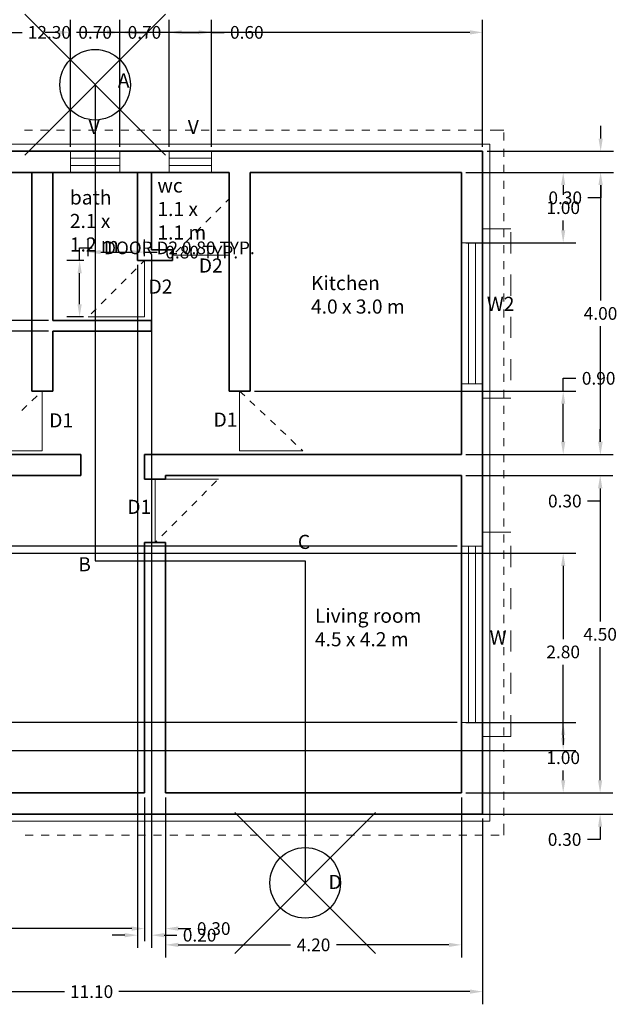
# Model space of a CAD drawing. Units: metres. Extents: x 37.9 to 70.9, y 22.7 to 44.8.
# Tile 2 of 4: x 44.9 to 53.4, y 22.7 to 36.7. Entities that reach past the tile are written whole.
import ezdxf

# ---------------------------------------------------------------- set-up
doc = ezdxf.new("R2010")
doc.units = ezdxf.units.M
doc.header["$LTSCALE"] = 50
doc.header["$MEASUREMENT"] = 0
doc.header["$PDMODE"] = 35
doc.header["$PDSIZE"] = -2
doc.linetypes.add('ACAD_ISO03W100', pattern=[30, 12, -18])
for name, color, linetype, lineweight in [('A-ANNO-DIMS', 2, 'Continuous', 18), ('A-ANNO-SYMB', 3, 'Continuous', 25), ('A-ANNO-TEXT', 7, 'Continuous', 18), ('A-AREA-IDEN', 7, 'Continuous', 18), ('A-DOOR', 4, 'Continuous', 18), ('A-FLOR-PLIN', 7, 'Continuous', 18), ('A-GLAZ', 4, 'Continuous', 18), ('A-ROOF-OVHD', 8, 'ACAD_ISO03W100', 13), ('A-WALL', 7, 'Continuous', 35)]:
    doc.layers.add(name, color=color, linetype=linetype, lineweight=lineweight)
doc.styles.get("Standard").update_dxf_attribs({"font": 'arial.ttf'})
doc.dimstyles.get("Standard").update_dxf_attribs({"dimtxt": 0.18, "dimasz": 0.18, "dimexe": 0.18, "dimexo": 0.0625, "dimgap": 0.09, "dimtad": 0, "dimtih": 1, "dimtoh": 1, "dimzin": 0, "dimdsep": 46, "dimtxsty": 'Standard', "dimcen": 0.09, "dimadec": 0, "dimazin": 0, "dimtfac": 1, "dimtofl": 0, "dimtmove": 0, "dimatfit": 3, "dimfxl": 1, "dimtolj": 1, "dimtzin": 0, "dimarcsym": 0})

# ---------------------------------------------------------------- blocks, each defined once
blk = doc.blocks.new('*D1')
at = {"layer": 'A-ANNO-DIMS', "color": 0, "linetype": 'ACAD_ISO03W100', "lineweight": -2, "transparency": 16777216}
for p, q in [((53.175, 34.98), (53.175, 35.16)), ((53.175, 34.32), (53.175, 34.14)), ((53.175, 34.14), (52.995, 34.14))]:
    blk.add_line(p, q, dxfattribs=at)
at = {"layer": 'A-ANNO-DIMS', "color": 0, "lineweight": -2, "transparency": 16777216}
for p, q in [((51.563, 34.8), (53.355, 34.8)), ((51.563, 34.5), (53.355, 34.5))]:
    blk.add_line(p, q, dxfattribs=at)
at = {"layer": 'A-ANNO-DIMS', "color": 0, "transparency": 16777216}
for points in [[(53.145, 34.98), (53.205, 34.98), (53.175, 34.8)], [(53.145, 34.32), (53.205, 34.32), (53.175, 34.5)]]:
    blk.add_solid(points, dxfattribs=at)
at = {"layer": 'Defpoints', "color": 0, "transparency": 16777216}
for p in [(51.5, 34.8), (51.5, 34.5), (53.175, 34.5)]:
    blk.add_point(p, dxfattribs=at)
at = {"layer": 'A-ANNO-DIMS', "color": 0, "transparency": 16777216, "insert": (52.672, 34.14), "char_height": 0.18, "attachment_point": 5}
blk.add_mtext('\\A1;0.30', dxfattribs=at)
blk = doc.blocks.new('*D2')
at = {"layer": 'A-ANNO-DIMS', "color": 0, "lineweight": -2, "transparency": 16777216}
for p, q in [((51.263, 34.5), (53.353, 34.5)), ((51.263, 30.5), (53.353, 30.5))]:
    blk.add_line(p, q, dxfattribs=at)
at = {"layer": 'A-ANNO-DIMS', "color": 0, "linetype": 'ACAD_ISO03W100', "lineweight": -2, "transparency": 16777216}
for p, q in [((53.173, 34.32), (53.173, 32.682)), ((53.173, 30.68), (53.173, 32.318))]:
    blk.add_line(p, q, dxfattribs=at)
at = {"layer": 'A-ANNO-DIMS', "color": 0, "transparency": 16777216}
for points in [[(53.143, 34.32), (53.203, 34.32), (53.173, 34.5)], [(53.143, 30.68), (53.203, 30.68), (53.173, 30.5)]]:
    blk.add_solid(points, dxfattribs=at)
at = {"layer": 'Defpoints', "color": 0, "transparency": 16777216}
for p in [(51.2, 34.5), (51.2, 30.5), (53.173, 30.5)]:
    blk.add_point(p, dxfattribs=at)
at = {"layer": 'A-ANNO-DIMS', "color": 0, "transparency": 16777216, "insert": (53.173, 32.5), "char_height": 0.18, "attachment_point": 5}
blk.add_mtext('\\A1;4.00', dxfattribs=at)
blk = doc.blocks.new('*D3')
at = {"layer": 'A-ANNO-DIMS', "color": 0, "linetype": 'ACAD_ISO03W100', "lineweight": -2, "transparency": 16777216}
for p, q in [((53.169, 30.68), (53.169, 30.86)), ((53.169, 30.02), (53.169, 29.84)), ((53.169, 29.84), (52.989, 29.84))]:
    blk.add_line(p, q, dxfattribs=at)
at = {"layer": 'A-ANNO-DIMS', "color": 0, "lineweight": -2, "transparency": 16777216}
for p, q in [((51.263, 30.5), (53.349, 30.5)), ((51.263, 30.2), (53.349, 30.2))]:
    blk.add_line(p, q, dxfattribs=at)
at = {"layer": 'A-ANNO-DIMS', "color": 0, "transparency": 16777216}
for points in [[(53.139, 30.68), (53.199, 30.68), (53.169, 30.5)], [(53.139, 30.02), (53.199, 30.02), (53.169, 30.2)]]:
    blk.add_solid(points, dxfattribs=at)
at = {"layer": 'Defpoints', "color": 0, "transparency": 16777216}
for p in [(51.2, 30.5), (51.2, 30.2), (53.169, 30.2)]:
    blk.add_point(p, dxfattribs=at)
at = {"layer": 'A-ANNO-DIMS', "color": 0, "transparency": 16777216, "insert": (52.666, 29.84), "char_height": 0.18, "attachment_point": 5}
blk.add_mtext('\\A1;0.30', dxfattribs=at)
blk = doc.blocks.new('*D4')
at = {"layer": 'A-ANNO-DIMS', "color": 0, "lineweight": -2, "transparency": 16777216}
for p, q in [((51.263, 30.2), (53.347, 30.2)), ((51.263, 25.7), (53.347, 25.7))]:
    blk.add_line(p, q, dxfattribs=at)
at = {"layer": 'A-ANNO-DIMS', "color": 0, "linetype": 'ACAD_ISO03W100', "lineweight": -2, "transparency": 16777216}
for p, q in [((53.167, 30.02), (53.167, 28.132)), ((53.167, 25.88), (53.167, 27.768))]:
    blk.add_line(p, q, dxfattribs=at)
at = {"layer": 'A-ANNO-DIMS', "color": 0, "transparency": 16777216}
for points in [[(53.137, 30.02), (53.197, 30.02), (53.167, 30.2)], [(53.137, 25.88), (53.197, 25.88), (53.167, 25.7)]]:
    blk.add_solid(points, dxfattribs=at)
at = {"layer": 'Defpoints', "color": 0, "transparency": 16777216}
for p in [(51.2, 30.2), (51.2, 25.7), (53.167, 25.7)]:
    blk.add_point(p, dxfattribs=at)
at = {"layer": 'A-ANNO-DIMS', "color": 0, "transparency": 16777216, "insert": (53.167, 27.95), "char_height": 0.18, "attachment_point": 5}
blk.add_mtext('\\A1;4.50', dxfattribs=at)
blk = doc.blocks.new('*D5')
at = {"layer": 'A-ANNO-DIMS', "color": 0, "linetype": 'ACAD_ISO03W100', "lineweight": -2, "transparency": 16777216}
for p, q in [((53.167, 25.88), (53.167, 26.06)), ((53.167, 25.22), (53.167, 25.04)), ((53.167, 25.04), (52.987, 25.04))]:
    blk.add_line(p, q, dxfattribs=at)
at = {"layer": 'A-ANNO-DIMS', "color": 0, "lineweight": -2, "transparency": 16777216}
for p, q in [((51.263, 25.7), (53.347, 25.7)), ((51.263, 25.4), (53.347, 25.4))]:
    blk.add_line(p, q, dxfattribs=at)
at = {"layer": 'A-ANNO-DIMS', "color": 0, "transparency": 16777216}
for points in [[(53.137, 25.88), (53.197, 25.88), (53.167, 25.7)], [(53.137, 25.22), (53.197, 25.22), (53.167, 25.4)]]:
    blk.add_solid(points, dxfattribs=at)
at = {"layer": 'Defpoints', "color": 0, "transparency": 16777216}
for p in [(51.2, 25.7), (51.2, 25.4), (53.167, 25.4)]:
    blk.add_point(p, dxfattribs=at)
at = {"layer": 'A-ANNO-DIMS', "color": 0, "transparency": 16777216, "insert": (52.663, 25.04), "char_height": 0.18, "attachment_point": 5}
blk.add_mtext('\\A1;0.30', dxfattribs=at)
blk = doc.blocks.new('*D6')
at = {"layer": 'A-ANNO-DIMS', "color": 0, "lineweight": -2, "transparency": 16777216}
for p, q in [((40.7, 25.637), (40.7, 23.597)), ((46.7, 25.637), (46.7, 23.597))]:
    blk.add_line(p, q, dxfattribs=at)
at = {"layer": 'A-ANNO-DIMS', "color": 0, "linetype": 'ACAD_ISO03W100', "lineweight": -2, "transparency": 16777216}
for p, q in [((40.88, 23.777), (43.376, 23.777)), ((46.52, 23.777), (44.024, 23.777))]:
    blk.add_line(p, q, dxfattribs=at)
at = {"layer": 'A-ANNO-DIMS', "color": 0, "transparency": 16777216}
for points in [[(40.88, 23.807), (40.88, 23.747), (40.7, 23.777)], [(46.52, 23.807), (46.52, 23.747), (46.7, 23.777)]]:
    blk.add_solid(points, dxfattribs=at)
at = {"layer": 'Defpoints', "color": 0, "transparency": 16777216}
for p in [(40.7, 25.7), (46.7, 25.7), (46.7, 23.777)]:
    blk.add_point(p, dxfattribs=at)
at = {"layer": 'A-ANNO-DIMS', "color": 0, "transparency": 16777216, "insert": (43.7, 23.777), "char_height": 0.18, "attachment_point": 5}
blk.add_mtext('\\A1;6.00', dxfattribs=at)
blk = doc.blocks.new('*D8')
at = {"layer": 'A-ANNO-DIMS', "color": 0, "lineweight": -2, "transparency": 16777216}
for p, q in [((46.7, 25.637), (46.7, 23.597)), ((47, 25.637), (47, 23.597))]:
    blk.add_line(p, q, dxfattribs=at)
at = {"layer": 'A-ANNO-DIMS', "color": 0, "linetype": 'ACAD_ISO03W100', "lineweight": -2, "transparency": 16777216}
for p, q in [((46.52, 23.777), (46.34, 23.777)), ((47.18, 23.777), (47.36, 23.777))]:
    blk.add_line(p, q, dxfattribs=at)
at = {"layer": 'A-ANNO-DIMS', "color": 0, "transparency": 16777216}
for points in [[(46.52, 23.807), (46.52, 23.747), (46.7, 23.777)], [(47.18, 23.807), (47.18, 23.747), (47, 23.777)]]:
    blk.add_solid(points, dxfattribs=at)
at = {"layer": 'Defpoints', "color": 0, "transparency": 16777216}
for p in [(46.7, 25.7), (47, 25.7), (47, 23.777)]:
    blk.add_point(p, dxfattribs=at)
at = {"layer": 'A-ANNO-DIMS', "color": 0, "transparency": 16777216, "insert": (47.683, 23.777), "char_height": 0.18, "attachment_point": 5}
blk.add_mtext('\\A1;0.30', dxfattribs=at)
blk = doc.blocks.new('*D9')
at = {"layer": 'A-ANNO-DIMS', "color": 0, "lineweight": -2, "transparency": 16777216}
for p, q in [((47, 25.637), (47, 23.366)), ((51.2, 25.637), (51.2, 23.366))]:
    blk.add_line(p, q, dxfattribs=at)
at = {"layer": 'A-ANNO-DIMS', "color": 0, "linetype": 'ACAD_ISO03W100', "lineweight": -2, "transparency": 16777216}
for p, q in [((47.18, 23.546), (48.773, 23.546)), ((51.02, 23.546), (49.427, 23.546))]:
    blk.add_line(p, q, dxfattribs=at)
at = {"layer": 'A-ANNO-DIMS', "color": 0, "transparency": 16777216}
for points in [[(47.18, 23.576), (47.18, 23.516), (47, 23.546)], [(51.02, 23.576), (51.02, 23.516), (51.2, 23.546)]]:
    blk.add_solid(points, dxfattribs=at)
at = {"layer": 'Defpoints', "color": 0, "transparency": 16777216}
for p in [(47, 25.7), (51.2, 25.7), (51.2, 23.546)]:
    blk.add_point(p, dxfattribs=at)
at = {"layer": 'A-ANNO-DIMS', "color": 0, "transparency": 16777216, "insert": (49.1, 23.546), "char_height": 0.18, "attachment_point": 5}
blk.add_mtext('\\A1;4.20', dxfattribs=at)
blk = doc.blocks.new('*D10')
at = {"layer": 'A-ANNO-DIMS', "color": 0, "lineweight": -2, "transparency": 16777216}
for p, q in [((40.4, 25.337), (40.4, 22.703)), ((51.5, 25.337), (51.5, 22.703))]:
    blk.add_line(p, q, dxfattribs=at)
at = {"layer": 'A-ANNO-DIMS', "color": 0, "linetype": 'ACAD_ISO03W100', "lineweight": -2, "transparency": 16777216}
for p, q in [((40.58, 22.883), (45.565, 22.883)), ((51.32, 22.883), (46.335, 22.883))]:
    blk.add_line(p, q, dxfattribs=at)
at = {"layer": 'A-ANNO-DIMS', "color": 0, "transparency": 16777216}
for points in [[(40.58, 22.913), (40.58, 22.853), (40.4, 22.883)], [(51.32, 22.913), (51.32, 22.853), (51.5, 22.883)]]:
    blk.add_solid(points, dxfattribs=at)
at = {"layer": 'Defpoints', "color": 0, "transparency": 16777216}
for p in [(40.4, 25.4), (51.5, 25.4), (51.5, 22.883)]:
    blk.add_point(p, dxfattribs=at)
at = {"layer": 'A-ANNO-DIMS', "color": 0, "transparency": 16777216, "insert": (45.95, 22.883), "char_height": 0.18, "attachment_point": 5}
blk.add_mtext('\\A1;11.10', dxfattribs=at)
blk = doc.blocks.new('WIN-2000-PLAN')
for p, q in [((0, 0.3), (0, 0)), ((2, 0.3), (2, 0)), ((0, 0.2), (2, 0.2)), ((0, 0.1), (2, 0.1))]:
    blk.add_line(p, q)
blk = doc.blocks.new('DOOR-800-PLAN')
for p, q in [((0, 0.8), (-0.046, 0.754)), ((0, 0), (0, 0.8)), ((-0.117, 0.683), (-0.188, 0.612)), ((-0.259, 0.541), (-0.329, 0.471)), ((-0.4, 0.4), (-0.471, 0.329)), ((-0.541, 0.259), (-0.612, 0.188)), ((-0.8, 0), (0, 0)), ((-0.683, 0.117), (-0.754, 0.046))]:
    blk.add_line(p, q)
blk = doc.blocks.new('*D17')
at = {"layer": 'A-ANNO-DIMS', "color": 0, "linetype": 'ACAD_ISO03W100', "lineweight": -2, "transparency": 16777216}
for p, q in [((45.78, 33.25), (45.78, 33.43)), ((45.78, 33.43), (45.96, 33.43)), ((45.78, 32.63), (45.78, 33.07))]:
    blk.add_line(p, q, dxfattribs=at)
at = {"layer": 'A-ANNO-DIMS', "color": 0, "lineweight": -2, "transparency": 16777216}
for p, q in [((45.838, 33.25), (45.6, 33.25)), ((45.837, 32.45), (45.6, 32.45))]:
    blk.add_line(p, q, dxfattribs=at)
at = {"layer": 'A-ANNO-DIMS', "color": 0, "transparency": 16777216}
for points in [[(45.75, 33.07), (45.81, 33.07), (45.78, 33.25)], [(45.75, 32.63), (45.81, 32.63), (45.78, 32.45)]]:
    blk.add_solid(points, dxfattribs=at)
at = {"layer": 'Defpoints', "color": 0, "transparency": 16777216}
for p in [(45.78, 33.25), (45.9, 33.25), (45.9, 32.45)]:
    blk.add_point(p, dxfattribs=at)
at = {"layer": 'A-ANNO-DIMS', "color": 0, "transparency": 16777216, "insert": (47.196, 33.43), "char_height": 0.18, "attachment_point": 5}
blk.add_mtext('\\A1;DOOR D2 0.80 TYP.', dxfattribs=at)
blk = doc.blocks.new('*D18')
at = {"layer": 'A-ANNO-DIMS', "color": 0, "lineweight": -2, "transparency": 16777216}
for p, q in [((45.9, 33.313), (45.9, 33.55)), ((46.7, 33.313), (46.7, 33.55))]:
    blk.add_line(p, q, dxfattribs=at)
at = {"layer": 'A-ANNO-DIMS', "color": 0, "linetype": 'ACAD_ISO03W100', "lineweight": -2, "transparency": 16777216}
for p, q in [((46.08, 33.37), (46.52, 33.37)), ((46.7, 33.37), (46.88, 33.37))]:
    blk.add_line(p, q, dxfattribs=at)
at = {"layer": 'A-ANNO-DIMS', "color": 0, "transparency": 16777216}
for points in [[(46.08, 33.4), (46.08, 33.34), (45.9, 33.37)], [(46.52, 33.4), (46.52, 33.34), (46.7, 33.37)]]:
    blk.add_solid(points, dxfattribs=at)
at = {"layer": 'Defpoints', "color": 0, "transparency": 16777216}
for p in [(45.9, 33.25), (46.7, 33.37), (46.7, 33.25)]:
    blk.add_point(p, dxfattribs=at)
at = {"layer": 'A-ANNO-DIMS', "color": 0, "transparency": 16777216, "insert": (47.513, 33.37), "char_height": 0.18, "attachment_point": 5}
blk.add_mtext('\\A1;0.80 TYP.', dxfattribs=at)
blk = doc.blocks.new('*D21')
at = {"layer": 'A-ANNO-DIMS', "color": 0, "lineweight": -2, "transparency": 16777216}
for p, q in [((45.65, 34.8625), (45.65, 36.665755)), ((46.35, 34.8625), (46.35, 36.665755))]:
    blk.add_line(p, q, dxfattribs=at)
at = {"layer": 'A-ANNO-DIMS', "color": 0, "linetype": 'ACAD_ISO03W100', "lineweight": -2, "transparency": 16777216}
for p, q in [((45.47, 36.485755), (45.29, 36.485755)), ((46.53, 36.485755), (46.71, 36.485755))]:
    blk.add_line(p, q, dxfattribs=at)
at = {"layer": 'A-ANNO-DIMS', "color": 0, "transparency": 16777216}
for points in [[(45.47, 36.515755), (45.47, 36.455755), (45.65, 36.485755)], [(46.53, 36.515755), (46.53, 36.455755), (46.35, 36.485755)]]:
    blk.add_solid(points, dxfattribs=at)
at = {"layer": 'Defpoints', "color": 0, "transparency": 16777216}
for p in [(46.35, 36.485755), (45.65, 34.8), (46.35, 34.8)]:
    blk.add_point(p, dxfattribs=at)
at = {"layer": 'A-ANNO-DIMS', "color": 0, "transparency": 16777216, "insert": (46, 36.485755), "char_height": 0.18, "attachment_point": 5}
blk.add_mtext('\\A1;0.70', dxfattribs=at)
blk = doc.blocks.new('*D22')
at = {"layer": 'A-ANNO-DIMS', "color": 0, "lineweight": -2, "transparency": 16777216}
for p, q in [((47.05, 34.862), (47.05, 36.666)), ((47.65, 34.862), (47.65, 36.666))]:
    blk.add_line(p, q, dxfattribs=at)
at = {"layer": 'A-ANNO-DIMS', "color": 0, "linetype": 'ACAD_ISO03W100', "lineweight": -2, "transparency": 16777216}
for p, q in [((47.23, 36.486), (47.47, 36.486)), ((47.65, 36.486), (47.83, 36.486))]:
    blk.add_line(p, q, dxfattribs=at)
at = {"layer": 'A-ANNO-DIMS', "color": 0, "transparency": 16777216}
for points in [[(47.23, 36.516), (47.23, 36.456), (47.05, 36.486)], [(47.47, 36.516), (47.47, 36.456), (47.65, 36.486)]]:
    blk.add_solid(points, dxfattribs=at)
at = {"layer": 'Defpoints', "color": 0, "transparency": 16777216}
for p in [(47.65, 36.486), (47.05, 34.8), (47.65, 34.8)]:
    blk.add_point(p, dxfattribs=at)
at = {"layer": 'A-ANNO-DIMS', "color": 0, "transparency": 16777216, "insert": (48.153, 36.486), "char_height": 0.18, "attachment_point": 5}
blk.add_mtext('\\A1;0.60', dxfattribs=at)
blk = doc.blocks.new('*D23')
at = {"layer": 'A-ANNO-DIMS', "color": 0, "lineweight": -2, "transparency": 16777216}
for p, q in [((46.35, 34.8625), (46.35, 36.665755)), ((47.05, 34.8625), (47.05, 36.665755))]:
    blk.add_line(p, q, dxfattribs=at)
at = {"layer": 'A-ANNO-DIMS', "color": 0, "linetype": 'ACAD_ISO03W100', "lineweight": -2, "transparency": 16777216}
for p, q in [((46.17, 36.485755), (45.99, 36.485755)), ((47.23, 36.485755), (47.41, 36.485755))]:
    blk.add_line(p, q, dxfattribs=at)
at = {"layer": 'A-ANNO-DIMS', "color": 0, "transparency": 16777216}
for points in [[(46.17, 36.515755), (46.17, 36.455755), (46.35, 36.485755)], [(47.23, 36.515755), (47.23, 36.455755), (47.05, 36.485755)]]:
    blk.add_solid(points, dxfattribs=at)
at = {"layer": 'Defpoints', "color": 0, "transparency": 16777216}
for p in [(47.05, 36.485755), (46.35, 34.8), (47.05, 34.8)]:
    blk.add_point(p, dxfattribs=at)
at = {"layer": 'A-ANNO-DIMS', "color": 0, "transparency": 16777216, "insert": (46.7, 36.485755), "char_height": 0.18, "attachment_point": 5}
blk.add_mtext('\\A1;0.70', dxfattribs=at)
blk = doc.blocks.new('*D24')
at = {"layer": 'A-ANNO-DIMS', "color": 0, "lineweight": -2, "transparency": 16777216}
for p, q in [((46.8, 33.337), (46.8, 23.503)), ((46.6, 33.188), (46.6, 23.503))]:
    blk.add_line(p, q, dxfattribs=at)
at = {"layer": 'A-ANNO-DIMS', "color": 0, "linetype": 'ACAD_ISO03W100', "lineweight": -2, "transparency": 16777216}
for p, q in [((46.42, 23.683), (46.24, 23.683)), ((46.98, 23.683), (47.16, 23.683))]:
    blk.add_line(p, q, dxfattribs=at)
at = {"layer": 'A-ANNO-DIMS', "color": 0, "transparency": 16777216}
for points in [[(46.42, 23.713), (46.42, 23.653), (46.6, 23.683)], [(46.98, 23.713), (46.98, 23.653), (46.8, 23.683)]]:
    blk.add_solid(points, dxfattribs=at)
at = {"layer": 'Defpoints', "color": 0, "transparency": 16777216}
for p in [(46.8, 33.4), (46.6, 33.25), (46.8, 23.683)]:
    blk.add_point(p, dxfattribs=at)
at = {"layer": 'A-ANNO-DIMS', "color": 0, "transparency": 16777216, "insert": (47.483, 23.683), "char_height": 0.18, "attachment_point": 5}
blk.add_mtext('\\A1;0.20', dxfattribs=at)
blk = doc.blocks.new('*D25')
at = {"layer": 'A-ANNO-DIMS', "color": 0, "linetype": 'ACAD_ISO03W100', "lineweight": -2, "transparency": 16777216}
for p, q in [((38.158, 32.58), (38.158, 32.76)), ((38.158, 32.76), (38.338, 32.76)), ((38.158, 32.07), (38.158, 31.89))]:
    blk.add_line(p, q, dxfattribs=at)
at = {"layer": 'A-ANNO-DIMS', "color": 0, "lineweight": -2, "transparency": 16777216}
for p, q in [((45.338, 32.4), (37.978, 32.4)), ((45.338, 32.25), (37.978, 32.25))]:
    blk.add_line(p, q, dxfattribs=at)
at = {"layer": 'A-ANNO-DIMS', "color": 0, "transparency": 16777216}
for points in [[(38.128, 32.58), (38.188, 32.58), (38.158, 32.4)], [(38.128, 32.07), (38.188, 32.07), (38.158, 32.25)]]:
    blk.add_solid(points, dxfattribs=at)
at = {"layer": 'Defpoints', "color": 0, "transparency": 16777216}
for p in [(38.158, 32.4), (45.4, 32.4), (45.4, 32.25)]:
    blk.add_point(p, dxfattribs=at)
at = {"layer": 'A-ANNO-DIMS', "color": 0, "transparency": 16777216, "insert": (38.662, 32.76), "char_height": 0.18, "attachment_point": 5}
blk.add_mtext('\\A1;0.15', dxfattribs=at)
blk = doc.blocks.new('*D26')
at = {"layer": 'A-ANNO-DIMS', "color": 0, "lineweight": -2, "transparency": 16777216}
for p, q in [((39.2, 34.862), (39.2, 36.666)), ((51.5, 34.862), (51.5, 36.666))]:
    blk.add_line(p, q, dxfattribs=at)
at = {"layer": 'A-ANNO-DIMS', "color": 0, "linetype": 'ACAD_ISO03W100', "lineweight": -2, "transparency": 16777216}
for p, q in [((39.38, 36.486), (44.965, 36.486)), ((51.32, 36.486), (45.735, 36.486))]:
    blk.add_line(p, q, dxfattribs=at)
at = {"layer": 'A-ANNO-DIMS', "color": 0, "transparency": 16777216}
for points in [[(39.38, 36.516), (39.38, 36.456), (39.2, 36.486)], [(51.32, 36.516), (51.32, 36.456), (51.5, 36.486)]]:
    blk.add_solid(points, dxfattribs=at)
at = {"layer": 'Defpoints', "color": 0, "transparency": 16777216}
for p in [(51.5, 36.486), (39.2, 34.8), (51.5, 34.8)]:
    blk.add_point(p, dxfattribs=at)
at = {"layer": 'A-ANNO-DIMS', "color": 0, "transparency": 16777216, "insert": (45.35, 36.486), "char_height": 0.18, "attachment_point": 5}
blk.add_mtext('\\A1;12.30', dxfattribs=at)
blk = doc.blocks.new('*D28')
at = {"layer": 'A-ANNO-DIMS', "color": 0, "lineweight": -2, "transparency": 16777216}
for p, q in [((40.763, 29.1), (52.823, 29.1)), ((40.763, 26.3), (52.823, 26.3))]:
    blk.add_line(p, q, dxfattribs=at)
at = {"layer": 'A-ANNO-DIMS', "color": 0, "linetype": 'ACAD_ISO03W100', "lineweight": -2, "transparency": 16777216}
for p, q in [((52.643, 28.92), (52.643, 27.882)), ((52.643, 26.48), (52.643, 27.518))]:
    blk.add_line(p, q, dxfattribs=at)
at = {"layer": 'A-ANNO-DIMS', "color": 0, "transparency": 16777216}
for points in [[(52.613, 28.92), (52.673, 28.92), (52.643, 29.1)], [(52.613, 26.48), (52.673, 26.48), (52.643, 26.3)]]:
    blk.add_solid(points, dxfattribs=at)
at = {"layer": 'Defpoints', "color": 0, "transparency": 16777216}
for p in [(40.7, 29.1), (52.643, 29.1), (40.7, 26.3)]:
    blk.add_point(p, dxfattribs=at)
at = {"layer": 'A-ANNO-DIMS', "color": 0, "transparency": 16777216, "insert": (52.643, 27.7), "char_height": 0.18, "attachment_point": 5}
blk.add_mtext('\\A1;2.80', dxfattribs=at)
blk = doc.blocks.new('*D30')
at = {"layer": 'A-ANNO-DIMS', "color": 0, "lineweight": -2, "transparency": 16777216}
for p, q in [((51.138, 29.2), (37.978, 29.2)), ((51.138, 26.7), (37.978, 26.7))]:
    blk.add_line(p, q, dxfattribs=at)
at = {"layer": 'A-ANNO-DIMS', "color": 0, "linetype": 'ACAD_ISO03W100', "lineweight": -2, "transparency": 16777216}
for p, q in [((38.158, 29.02), (38.158, 28.132)), ((38.158, 26.88), (38.158, 27.768))]:
    blk.add_line(p, q, dxfattribs=at)
at = {"layer": 'A-ANNO-DIMS', "color": 0, "transparency": 16777216}
for points in [[(38.128, 29.02), (38.188, 29.02), (38.158, 29.2)], [(38.128, 26.88), (38.188, 26.88), (38.158, 26.7)]]:
    blk.add_solid(points, dxfattribs=at)
at = {"layer": 'Defpoints', "color": 0, "transparency": 16777216}
for p in [(38.158, 29.2), (51.2, 29.2), (51.2, 26.7)]:
    blk.add_point(p, dxfattribs=at)
at = {"layer": 'A-ANNO-DIMS', "color": 0, "transparency": 16777216, "insert": (38.158, 27.95), "char_height": 0.18, "attachment_point": 5}
blk.add_mtext('\\A1;2.50', dxfattribs=at)
blk = doc.blocks.new('*D31')
at = {"layer": 'A-ANNO-DIMS', "color": 0, "lineweight": -2, "transparency": 16777216}
for p, q in [((51.263, 26.7), (52.823, 26.7)), ((51.263, 25.7), (52.823, 25.7))]:
    blk.add_line(p, q, dxfattribs=at)
at = {"layer": 'A-ANNO-DIMS', "color": 0, "linetype": 'ACAD_ISO03W100', "lineweight": -2, "transparency": 16777216}
for p, q in [((52.643, 26.52), (52.643, 26.382)), ((52.643, 25.88), (52.643, 26.018))]:
    blk.add_line(p, q, dxfattribs=at)
at = {"layer": 'A-ANNO-DIMS', "color": 0, "transparency": 16777216}
for points in [[(52.613, 26.52), (52.673, 26.52), (52.643, 26.7)], [(52.613, 25.88), (52.673, 25.88), (52.643, 25.7)]]:
    blk.add_solid(points, dxfattribs=at)
at = {"layer": 'Defpoints', "color": 0, "transparency": 16777216}
for p in [(51.2, 26.7), (52.643, 26.7), (51.2, 25.7)]:
    blk.add_point(p, dxfattribs=at)
at = {"layer": 'A-ANNO-DIMS', "color": 0, "transparency": 16777216, "insert": (52.643, 26.2), "char_height": 0.18, "attachment_point": 5}
blk.add_mtext('\\A1;1.00', dxfattribs=at)
blk = doc.blocks.new('*D32')
at = {"layer": 'A-ANNO-DIMS', "color": 0, "lineweight": -2, "transparency": 16777216}
for p, q in [((51.263, 34.5), (52.823, 34.5)), ((51.263, 33.5), (52.823, 33.5))]:
    blk.add_line(p, q, dxfattribs=at)
at = {"layer": 'A-ANNO-DIMS', "color": 0, "linetype": 'ACAD_ISO03W100', "lineweight": -2, "transparency": 16777216}
for p, q in [((52.643, 34.32), (52.643, 34.182)), ((52.643, 33.68), (52.643, 33.818))]:
    blk.add_line(p, q, dxfattribs=at)
at = {"layer": 'A-ANNO-DIMS', "color": 0, "transparency": 16777216}
for points in [[(52.613, 34.32), (52.673, 34.32), (52.643, 34.5)], [(52.613, 33.68), (52.673, 33.68), (52.643, 33.5)]]:
    blk.add_solid(points, dxfattribs=at)
at = {"layer": 'Defpoints', "color": 0, "transparency": 16777216}
for p in [(51.2, 34.5), (51.2, 33.5), (52.643, 33.5)]:
    blk.add_point(p, dxfattribs=at)
at = {"layer": 'A-ANNO-DIMS', "color": 0, "transparency": 16777216, "insert": (52.643, 34), "char_height": 0.18, "attachment_point": 5}
blk.add_mtext('\\A1;1.00', dxfattribs=at)
blk = doc.blocks.new('*D33')
at = {"layer": 'A-ANNO-DIMS', "color": 0, "linetype": 'ACAD_ISO03W100', "lineweight": -2, "transparency": 16777216}
for p, q in [((52.643, 31.4), (52.643, 31.58)), ((52.643, 31.58), (52.823, 31.58)), ((52.643, 30.68), (52.643, 31.22))]:
    blk.add_line(p, q, dxfattribs=at)
at = {"layer": 'A-ANNO-DIMS', "color": 0, "lineweight": -2, "transparency": 16777216}
for p, q in [((48.263, 31.4), (52.823, 31.4)), ((51.263, 30.5), (52.823, 30.5))]:
    blk.add_line(p, q, dxfattribs=at)
at = {"layer": 'A-ANNO-DIMS', "color": 0, "transparency": 16777216}
for points in [[(52.613, 31.22), (52.673, 31.22), (52.643, 31.4)], [(52.613, 30.68), (52.673, 30.68), (52.643, 30.5)]]:
    blk.add_solid(points, dxfattribs=at)
at = {"layer": 'Defpoints', "color": 0, "transparency": 16777216}
for p in [(48.2, 31.4), (52.643, 31.4), (51.2, 30.5)]:
    blk.add_point(p, dxfattribs=at)
at = {"layer": 'A-ANNO-DIMS', "color": 0, "transparency": 16777216, "insert": (53.146, 31.58), "char_height": 0.18, "attachment_point": 5}
blk.add_mtext('\\A1;0.90', dxfattribs=at)

msp = doc.modelspace()

# ---------------------------------------------------------------- linework, layer by layer
at = {"layer": 'A-ANNO-SYMB'}
for p, q in [((46, 35.7433), (46, 28.9936)), ((46, 28.9936), (48.9811, 28.9936)), ((48.9811, 28.9936), (48.9811, 24.4253))]:
    msp.add_line(p, q, dxfattribs=at)
for p in [(46, 35.7433), (48.9811, 24.4253)]:
    msp.add_point(p, dxfattribs=at)
at = {"layer": 'A-DOOR'}
for p, q in [((45.1038, 31.2619), (45.1765, 31.3306)), ((45.25, 31.4), (45.25, 30.55)), ((48.05, 31.4), (48.05, 30.55)), ((48.1235, 31.3306), (48.05, 31.4)), ((44.9583, 31.1245), (45.0311, 31.1932)), ((48.2689, 31.1932), (48.1962, 31.2619)), ((48.4144, 31.0558), (48.3417, 31.1245)), ((48.5599, 30.9185), (48.4871, 30.9871)), ((48.7053, 30.7811), (48.6326, 30.8498)), ((48.8508, 30.6437), (48.7781, 30.7124)), ((45.25, 30.55), (44.35, 30.55)), ((48.05, 30.55), (48.95, 30.55)), ((48.95, 30.55), (48.9235, 30.575)), ((46.85, 29.25), (46.85, 30.15)), ((46.85, 30.15), (47.75, 30.15)), ((47.7243, 30.1243), (47.6536, 30.0536)), ((47.5828, 29.9828), (47.5121, 29.9121)), ((47.4414, 29.8414), (47.3707, 29.7707)), ((47.3, 29.7), (47.2293, 29.6293)), ((47.1586, 29.5586), (47.0879, 29.4879)), ((47.0172, 29.4172), (46.9464, 29.3464)), ((46.8757, 29.2757), (46.85, 29.25))]:
    msp.add_line(p, q, dxfattribs=at)
at = {"layer": 'A-FLOR-PLIN'}
msp.add_lwpolyline([(39.1, 30.1), (39.1, 34.9), (51.6, 34.9), (51.6, 25.3), (40.3, 25.3), (40.3, 29.3)], dxfattribs=at)
at = {"layer": 'A-GLAZ'}
for p, q in [((45.65, 34.5), (45.65, 34.8)), ((46.35, 34.5), (46.35, 34.8)), ((47.05, 34.5), (47.05, 34.8)), ((47.65, 34.5), (47.65, 34.8)), ((45.65, 34.7), (46.35, 34.7)), ((47.05, 34.7), (47.65, 34.7)), ((45.65, 34.6), (46.35, 34.6)), ((47.05, 34.6), (47.65, 34.6)), ((51.2, 29.2), (51.5, 29.2)), ((51.3, 29.2), (51.3, 26.7)), ((51.4, 29.2), (51.4, 26.7)), ((51.2, 26.7), (51.5, 26.7))]:
    msp.add_line(p, q, dxfattribs=at)
at = {"layer": 'A-ROOF-OVHD'}
for p, q in [((51.5, 33.5), (51.5, 33.7)), ((51.5, 31.5), (51.5, 31.3)), ((51.5, 29.2), (51.5, 29.4)), ((51.5, 29.4), (51.9, 29.4)), ((51.9, 29.2044), (51.9, 28.9044)), ((51.9, 28.6044), (51.9, 28.3044)), ((51.9, 28.0044), (51.9, 27.7044)), ((51.9, 27.4044), (51.9, 27.1044)), ((51.9, 26.8044), (51.9, 26.5)), ((51.9, 26.5), (51.5, 26.5))]:
    msp.add_line(p, q, dxfattribs=at)
for points in [[(44.9957, 35.1), (45.1097, 35.1)], [(45.2237, 35.1), (45.3377, 35.1)], [(45.4517, 35.1), (45.5657, 35.1)], [(45.6797, 35.1), (45.7937, 35.1)], [(45.9077, 35.1), (46.0217, 35.1)], [(46.1357, 35.1), (46.2497, 35.1)], [(46.3637, 35.1), (46.4777, 35.1)], [(46.5917, 35.1), (46.7057, 35.1)], [(46.8197, 35.1), (46.9337, 35.1)], [(47.0477, 35.1), (47.1617, 35.1)], [(47.2757, 35.1), (47.3897, 35.1)], [(47.5037, 35.1), (47.6177, 35.1)], [(47.7317, 35.1), (47.8457, 35.1)], [(47.9597, 35.1), (48.0737, 35.1)], [(48.1877, 35.1), (48.3017, 35.1)], [(48.4157, 35.1), (48.5297, 35.1)], [(48.6437, 35.1), (48.7577, 35.1)], [(48.8717, 35.1), (48.9857, 35.1)], [(49.0997, 35.1), (49.2137, 35.1)], [(49.3277, 35.1), (49.4417, 35.1)], [(49.5557, 35.1), (49.6697, 35.1)], [(49.7837, 35.1), (49.8977, 35.1)], [(50.0117, 35.1), (50.1257, 35.1)], [(50.2397, 35.1), (50.3537, 35.1)], [(50.4677, 35.1), (50.5817, 35.1)], [(50.6957, 35.1), (50.8097, 35.1)], [(50.9237, 35.1), (51.0377, 35.1)], [(51.1517, 35.1), (51.2657, 35.1)], [(51.3797, 35.1), (51.4937, 35.1)], [(51.6077, 35.1), (51.8, 35.1)], [(51.8, 35.0643), (51.8, 34.9503)], [(51.8, 34.8363), (51.8, 34.7223)], [(51.8, 34.6083), (51.8, 34.4943)], [(51.8, 34.3803), (51.8, 34.2663)], [(51.8, 34.1523), (51.8, 34.0383)], [(51.8, 33.9243), (51.8, 33.8103)], [(51.5, 33.7), (51.9, 33.7)], [(51.8, 33.6963), (51.8, 33.5822)], [(51.9, 33.6519), (51.9, 33.3519)], [(51.8, 33.4682), (51.8, 33.3542)], [(51.8, 33.2402), (51.8, 33.1262)], [(51.8, 33.0122), (51.8, 32.8982)], [(51.9, 33.0519), (51.9, 32.7519)], [(51.8, 32.7842), (51.8, 32.6702)], [(51.8, 32.5562), (51.8, 32.4422)], [(51.9, 32.4519), (51.9, 32.1519)], [(51.8, 32.3282), (51.8, 32.2142)], [(51.8, 32.1002), (51.8, 31.9862)], [(51.8, 31.8722), (51.8, 31.7582)], [(51.9, 31.8519), (51.9, 31.5519)], [(51.8, 31.6442), (51.8, 31.5302)], [(51.8, 31.4162), (51.8, 31.3022)], [(51.9, 31.3), (51.5, 31.3)], [(51.8, 31.1882), (51.8, 31.0742)], [(51.8, 30.9602), (51.8, 30.8462)], [(51.8, 30.7322), (51.8, 30.6182)], [(51.8, 30.5042), (51.8, 30.3902)], [(51.8, 30.2762), (51.8, 30.1622)], [(51.8, 30.0482), (51.8, 29.9342)], [(51.8, 29.8202), (51.8, 29.7062)], [(51.8, 29.5922), (51.8, 29.4782)], [(51.8, 29.3642), (51.8, 29.2502)], [(51.8, 29.1362), (51.8, 29.0222)], [(51.8, 28.9082), (51.8, 28.7942)], [(51.8, 28.6802), (51.8, 28.5662)], [(51.8, 28.4522), (51.8, 28.3382)], [(51.8, 28.2242), (51.8, 28.1102)], [(51.8, 27.9962), (51.8, 27.8822)], [(51.8, 27.7682), (51.8, 27.6542)], [(51.8, 27.5402), (51.8, 27.4262)], [(51.8, 27.3122), (51.8, 27.1982)], [(51.8, 27.0842), (51.8, 26.9702)], [(51.8, 26.8562), (51.8, 26.7422)], [(51.8, 26.6282), (51.8, 26.5142)], [(51.8, 26.4002), (51.8, 26.2862)], [(51.8, 26.1722), (51.8, 26.0582)], [(51.8, 25.9442), (51.8, 25.8302)], [(51.8, 25.7162), (51.8, 25.6022)], [(51.8, 25.4882), (51.8, 25.3742)], [(51.8, 25.2602), (51.8, 25.1)], [(45.1201, 25.1), (45.0061, 25.1)], [(45.3481, 25.1), (45.2341, 25.1)], [(45.5761, 25.1), (45.4621, 25.1)], [(45.8041, 25.1), (45.6901, 25.1)], [(46.0321, 25.1), (45.9181, 25.1)], [(46.2601, 25.1), (46.1461, 25.1)], [(46.4881, 25.1), (46.3741, 25.1)], [(46.7161, 25.1), (46.6021, 25.1)], [(46.9441, 25.1), (46.8301, 25.1)], [(47.1721, 25.1), (47.0581, 25.1)], [(47.4001, 25.1), (47.2861, 25.1)], [(47.6281, 25.1), (47.5141, 25.1)], [(47.8561, 25.1), (47.7421, 25.1)], [(48.0841, 25.1), (47.9701, 25.1)], [(48.3121, 25.1), (48.1981, 25.1)], [(48.5401, 25.1), (48.4261, 25.1)], [(48.7681, 25.1), (48.6541, 25.1)], [(48.9961, 25.1), (48.8821, 25.1)], [(49.2241, 25.1), (49.1101, 25.1)], [(49.4521, 25.1), (49.3381, 25.1)], [(49.6801, 25.1), (49.5661, 25.1)], [(49.9081, 25.1), (49.7941, 25.1)], [(50.1361, 25.1), (50.0221, 25.1)], [(50.3641, 25.1), (50.2501, 25.1)], [(50.5921, 25.1), (50.4781, 25.1)], [(50.8202, 25.1), (50.7062, 25.1)], [(51.0482, 25.1), (50.9342, 25.1)], [(51.2762, 25.1), (51.1622, 25.1)], [(51.5042, 25.1), (51.3902, 25.1)], [(51.7322, 25.1), (51.6182, 25.1)]]:
    msp.add_lwpolyline(points, dxfattribs=at)
at = {"layer": 'A-WALL'}
for p, q in [((39.2, 34.8), (51.5, 34.8)), ((51.5, 34.8), (51.5, 25.4)), ((42.1, 34.5), (47.9, 34.5)), ((45.1, 34.5), (45.1, 31.4)), ((45.4, 34.5), (45.4, 32.4)), ((46.6, 34.5), (46.6, 33.25)), ((46.8, 34.5), (46.8, 33.4)), ((47.9, 34.5), (47.9, 31.4)), ((48.2, 34.5), (48.2, 31.4)), ((48.2, 34.5), (51.2, 34.5)), ((51.2, 34.5), (51.2, 30.5)), ((47.1, 33.4), (46.8, 33.4)), ((47.1, 33.4), (47.1, 33.25)), ((47.1, 33.25), (46.6, 33.25)), ((46.8, 32.4), (45.4, 32.4)), ((46.8, 32.4), (46.8, 32.25)), ((46.8, 32.25), (45.4, 32.25)), ((45.4, 32.25), (45.4, 31.4)), ((45.4, 31.4), (45.1, 31.4)), ((48.2, 31.4), (47.9, 31.4)), ((45.7966, 30.5), (42.1, 30.5)), ((45.7966, 30.5), (45.7966, 30.2)), ((51.2, 30.5), (46.7, 30.5)), ((46.7, 30.5), (46.7, 30.15)), ((45.7966, 30.2), (41.75, 30.2)), ((51.2, 30.2), (47, 30.2)), ((47, 30.2), (47, 30.15)), ((51.2, 30.2), (51.2, 25.7)), ((47, 30.15), (46.7, 30.15)), ((47, 29.25), (46.7, 29.25)), ((46.7, 29.25), (46.7, 25.7)), ((47, 29.25), (47, 25.7)), ((46.7, 25.7), (40.7, 25.7)), ((51.2, 25.7), (47, 25.7)), ((51.5, 25.4), (40.4, 25.4))]:
    msp.add_line(p, q, dxfattribs=at)

# ---------------------------------------------------------------- block references
at = {"layer": 'A-DOOR'}
msp.add_blockref('DOOR-800-PLAN', (47.9, 33.325), dxfattribs=at)
at = {"layer": 'A-DOOR', "rotation": 359.9974951750775}
msp.add_blockref('DOOR-800-PLAN', (46.7, 32.45), dxfattribs=at)
at = {"layer": 'A-GLAZ', "rotation": 89.99999999999946}
msp.add_blockref('WIN-2000-PLAN', (51.5, 31.5), dxfattribs=at)

# ---------------------------------------------------------------- texts
at = {"layer": 'A-ANNO-SYMB', "char_height": 0.2, "attachment_point": 1}
for s, insert in [('A', (46.3215, 35.9031)), ('C', (48.877, 29.3605)), ('B', (45.7602, 29.0437)), ('D', (49.3122, 24.5382))]:
    msp.add_mtext_dynamic_manual_height_columns(s, width=0.601082, gutter_width=1, heights=[0], dxfattribs=dict(at, insert=insert))
at = {"layer": 'A-ANNO-TEXT', "char_height": 0.2, "attachment_point": 1}
for s, insert in [('V', (45.9077, 35.2433)), ('V', (47.3149, 35.2433)), ('D2', (47.4717, 33.2794)), ('D2', (46.7578, 32.9809)), ('W2', (51.5597, 32.736)), ('D1', (45.3481, 31.0838)), ('D1', (47.6806, 31.0948)), ('D1', (46.4572, 29.8576)), ('W', (51.6, 28.0047))]:
    msp.add_mtext_dynamic_manual_height_columns(s, width=0.601082, gutter_width=1, heights=[0], dxfattribs=dict(at, insert=insert))
at = {"layer": 'A-AREA-IDEN', "char_height": 0.2, "attachment_point": 1}
for s, width, insert in [('wc\\P1.1 x 1.1 m', 0.976285, (46.8841, 34.4147)), ('bath\\P2.1 x 1.2 m', 0.722747, (45.6415, 34.245)), ('Kitchen\\P4.0 x 3.0 m', 1.544693, (49.0636, 33.0313)), ('Living room\\P4.5 x 4.2 m', 1.544693, (49.1194, 28.3135))]:
    msp.add_mtext_dynamic_manual_height_columns(s, width=width, gutter_width=1, heights=[0], dxfattribs=dict(at, insert=insert))

# ---------------------------------------------------------------- dimensions: what is measured, and where the dimension line sits
at = {"layer": 'A-ANNO-DIMS'}
for base, p1, p2, override, picture, middle in [((51.5, 36.4858), (39.2, 34.8), (51.5, 34.8), {"dimdec": 2, "dimlfac": 1, "dimrnd": 0, "dimzin": 0, "dimdsep": 46, "dimlunit": 2}, '*D26', (45.35, 36.4858)), ((46.35, 36.4858), (45.65, 34.8), (46.35, 34.8), {"dimdec": 2, "dimlfac": 1, "dimrnd": 0, "dimzin": 0, "dimdsep": 46, "dimlunit": 2}, '*D21', (46, 36.4858)), ((47.05, 36.4858), (46.35, 34.8), (47.05, 34.8), {"dimdec": 2, "dimlfac": 1, "dimrnd": 0, "dimzin": 0, "dimdsep": 46, "dimlunit": 2}, '*D23', (46.7, 36.4858)), ((47.65, 36.4858), (47.05, 34.8), (47.65, 34.8), {"dimdec": 2, "dimlfac": 1, "dimrnd": 0, "dimzin": 0, "dimdsep": 46, "dimlunit": 2}, '*D22', (48.1535, 36.4858)), ((46.8, 23.6828), (46.6, 33.25), (46.8, 33.4), {"dimdec": 2, "dimlfac": 1, "dimrnd": 0, "dimzin": 0, "dimdsep": 46, "dimlunit": 2}, '*D24', (47.4835, 23.6828)), ((46.7, 23.7769), (40.7, 25.7), (46.7, 25.7), {"dimclrd": 0, "dimclre": 0, "dimclrt": 0}, '*D6', (43.7, 23.7769)), ((47, 23.7769), (46.7, 25.7), (47, 25.7), {"dimclrd": 0, "dimclre": 0, "dimclrt": 0}, '*D8', (47.6835, 23.7769)), ((51.2, 23.5457), (47, 25.7), (51.2, 25.7), {"dimclrd": 0, "dimclre": 0, "dimclrt": 0}, '*D9', (49.1, 23.5457)), ((51.5, 22.8831), (40.4, 25.4), (51.5, 25.4), {"dimclrd": 0, "dimclre": 0, "dimclrt": 0}, '*D10', (45.95, 22.8831))]:
    dim = msp.add_linear_dim(base=base, p1=p1, p2=p2, dimstyle='Standard', override=override, dxfattribs=at)
    dim.commit()
    dim.dimension.update_dxf_attribs({"geometry": picture, "text_midpoint": middle})
for base, p1, p2, override, picture, middle in [((53.1755, 34.5), (51.5, 34.8), (51.5, 34.5), {"dimclrd": 0, "dimclre": 0, "dimclrt": 0}, '*D1', (52.672, 34.14)), ((53.1726, 30.5), (51.2, 34.5), (51.2, 30.5), {"dimclrd": 0, "dimclre": 0, "dimclrt": 0}, '*D2', (53.1726, 32.5)), ((52.6425, 33.5), (51.2, 34.5), (51.2, 33.5), {"dimdec": 2, "dimlfac": 1, "dimrnd": 0, "dimzin": 0, "dimdsep": 46, "dimlunit": 2}, '*D32', (52.6425, 34)), ((38.1575, 32.4), (45.4, 32.25), (45.4, 32.4), {"dimdec": 2, "dimlfac": 1, "dimrnd": 0, "dimzin": 0, "dimdsep": 46, "dimlunit": 2}, '*D25', (38.662, 32.76)), ((52.6425, 31.4), (51.2, 30.5), (48.2, 31.4), {"dimdec": 2, "dimlfac": 1, "dimrnd": 0, "dimzin": 0, "dimdsep": 46, "dimlunit": 2}, '*D33', (53.146, 31.58)), ((53.1693, 30.2), (51.2, 30.5), (51.2, 30.2), {"dimclrd": 0, "dimclre": 0, "dimclrt": 0}, '*D3', (52.6658, 29.84)), ((53.167, 25.7), (51.2, 30.2), (51.2, 25.7), {"dimclrd": 0, "dimclre": 0, "dimclrt": 0}, '*D4', (53.167, 27.95)), ((38.1575, 29.2), (51.2, 26.7), (51.2, 29.2), {"dimdec": 2, "dimlfac": 1, "dimrnd": 0, "dimzin": 0, "dimdsep": 46, "dimlunit": 2}, '*D30', (38.1575, 27.95)), ((52.6425, 29.1), (40.7, 26.3), (40.7, 29.1), {"dimdec": 2, "dimlfac": 1, "dimrnd": 0, "dimzin": 0, "dimdsep": 46, "dimlunit": 2}, '*D28', (52.6425, 27.7)), ((52.6425, 26.7), (51.2, 25.7), (51.2, 26.7), {"dimdec": 2, "dimlfac": 1, "dimrnd": 0, "dimzin": 0, "dimdsep": 46, "dimlunit": 2}, '*D31', (52.6425, 26.2)), ((53.167, 25.4), (51.2, 25.7), (51.2, 25.4), {"dimclrd": 0, "dimclre": 0, "dimclrt": 0}, '*D5', (52.6635, 25.04))]:
    dim = msp.add_linear_dim(base=base, p1=p1, p2=p2, angle=90, dimstyle='Standard', override=override, dxfattribs=at)
    dim.commit()
    dim.dimension.update_dxf_attribs({"geometry": picture, "text_midpoint": middle})
for base, p1, p2, angle, text, picture, middle in [((45.78, 33.2501), (45.9, 32.45), (45.9, 33.2501), 89.9975, 'DOOR D2 <> TYP.', '*D17', (47.1963, 33.4301)), ((46.7, 33.3701), (45.9, 33.2501), (46.7, 33.25), 359.9975, '<> TYP.', '*D18', (47.513, 33.37))]:
    dim = msp.add_linear_dim(base=base, p1=p1, p2=p2, angle=angle, text=text, dimstyle='Standard', override={"dimdec": 2, "dimlfac": 1, "dimrnd": 0, "dimzin": 0, "dimdsep": 46, "dimlunit": 2}, dxfattribs=at)
    dim.commit()
    dim.dimension.update_dxf_attribs({"geometry": picture, "text_midpoint": middle})

doc.saveas('drawing.dxf')
